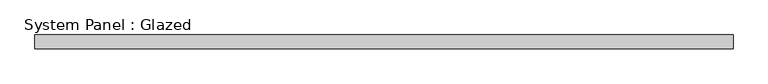
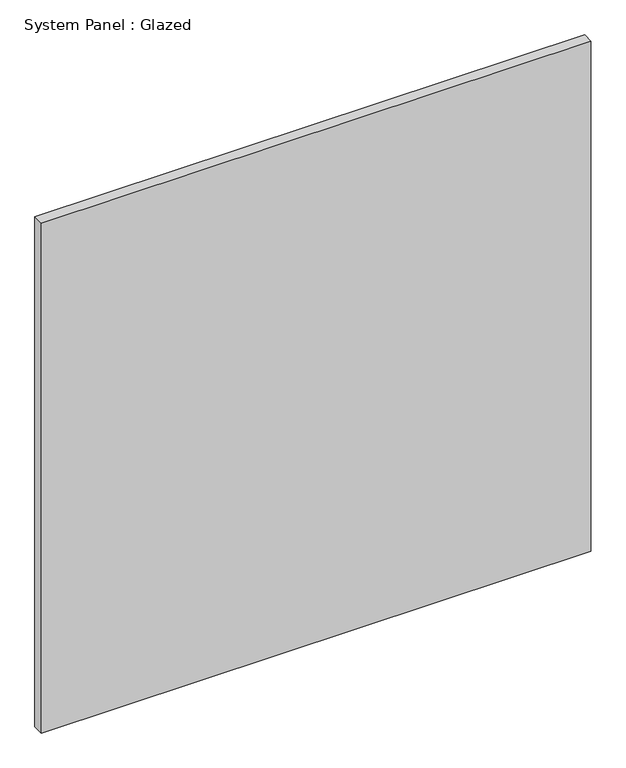
"""IFC4 building model written with IfcOpenShell, lengths in millimetres: plate geometry, System Panel : Glazed."""

from ifc_helpers import new_model, si_unit, origin, origin_with_axes, place, context, project, spatial, polyline, outline, extrude, source, transform, mapped, element, save


def system_panel_glazed_4e3b5d9d(model_context):
    return source(origin(), model_context, "Body", "SweptSolid", [
        extrude(outline(polyline([(641.35, 19.05), (-641.35, 19.05), (-641.35, 44.45), (641.35, 44.45), (641.35, 19.05)])), origin_with_axes(), (0.0, 0.0, 1.0), 1258.0860761),
    ])


if __name__ == "__main__":
    model = new_model("IFC4")
    model_context = context("Model", 3, world=origin())
    ifc_project = project(units=[si_unit("LENGTHUNIT", "METRE", prefix="MILLI")], contexts=[model_context])
    site = spatial("IfcSite", under=ifc_project)
    building = spatial("IfcBuilding", under=site)
    placement = place(None, origin())
    system_panel_glazed_shape = system_panel_glazed_4e3b5d9d(model_context)
    element("IfcPlate", 1, ObjectType="System Panel : Glazed", at=placement, inside=building, context=model_context, shape_type="MappedRepresentation", body=[
        mapped(system_panel_glazed_shape, transform((0.0, 0.0, 0.0), x_axis=(1.0, 0.0, 0.0), y_axis=(0.0, 1.0, 0.0), z_axis=(0.0, 0.0, 1.0))),
    ])
    save(model, "model.ifc")

# Revit data of these elements
# Type "System Panel : Glazed"
#   Construction Type Id = "GSP4R"
#   Analytic Construction = "1/8 in Pilkington single glazing"
#   Visual Light Transmittance = 0.9
#   Solar Heat Gain Coefficient = 0.86
#   Heat Transfer Coefficient (U) = 1.18115 BTU/(h·ft²·°F)
#   Define Thermal Properties by = 1
# Element 1 (IfcPlate, "System Panel : Glazed")
#   Materials on its faces: "Glass"
# Materials
#   "Glass": class "Glass", colour RGB 0 128 192, transparency 0.75, Description = "Soda Lime Glass", Cost = 0
